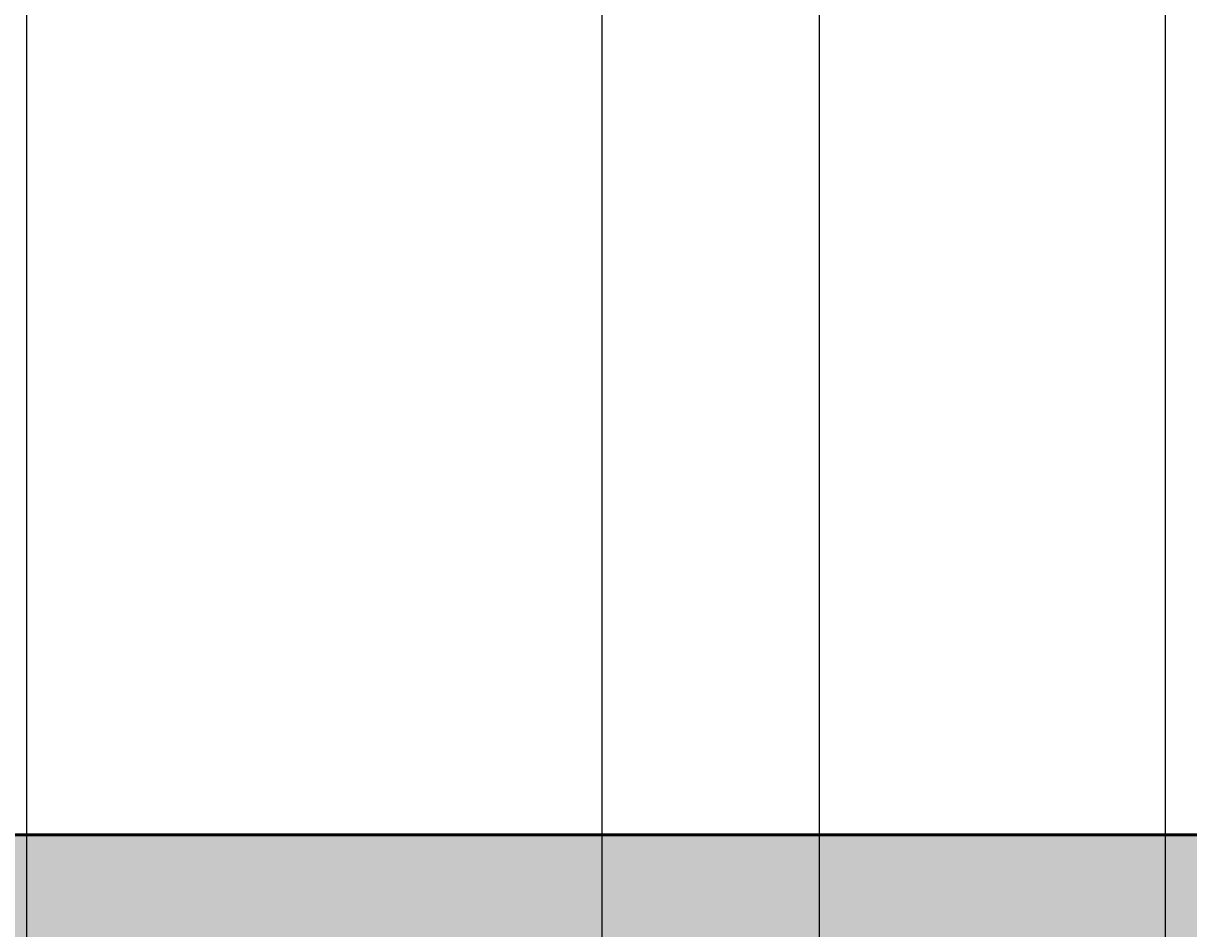
# Model space of a CAD drawing. Units: inches. Extents: x 2231 to 2461, y 2045 to 2455.
# Tile 81 of 95: x 2384 to 2409, y 2333 to 2352. Entities that reach past the tile are written whole.
import ezdxf

# ---------------------------------------------------------------- set-up
doc = ezdxf.new("R2010")
doc.units = ezdxf.units.IN
doc.layers.add('A-ANNO-DIMS', color=2, linetype='Continuous', lineweight=18)
doc.layers.add('A-WALL', color=7, linetype='Continuous', lineweight=50)
doc.layers.add('A-WALL-PATT', color=18, linetype='Continuous', lineweight=13, true_color=0x000000)
doc.styles.get("Standard").update_dxf_attribs({"font": 'arial.ttf'})
doc.dimstyles.get("Standard").update_dxf_attribs({"dimtxt": 0.18, "dimasz": 0.18, "dimexe": 0.18, "dimexo": 0.0625, "dimgap": 0.09, "dimtad": 0, "dimtih": 1, "dimtoh": 1, "dimdec": 4, "dimzin": 0, "dimdsep": 46, "dimtxsty": 'Standard', "dimcen": 0.09, "dimadec": 0, "dimazin": 0, "dimtfac": 1, "dimtdec": 4, "dimtofl": 0, "dimtmove": 0, "dimatfit": 3, "dimfxl": 1, "dimtolj": 1, "dimtzin": 0, "dimarcsym": 0})

# ---------------------------------------------------------------- blocks, each defined once
blk = doc.blocks.new('*D42')
at = {"layer": 'A-ANNO-DIMS', "color": 0, "lineweight": -2, "transparency": 16777216}
for p, q in [((2396.794, 2286.895), (2396.794, 2454.645)), ((2432.794, 2286.895), (2432.794, 2454.645)), ((2396.974, 2454.465), (2414.575, 2454.465)), ((2432.614, 2454.465), (2415.012, 2454.465))]:
    blk.add_line(p, q, dxfattribs=at)
at = {"layer": 'A-ANNO-DIMS', "color": 0, "transparency": 16777216}
for points in [[(2396.974, 2454.495), (2396.974, 2454.435), (2396.794, 2454.465)], [(2432.614, 2454.495), (2432.614, 2454.435), (2432.794, 2454.465)]]:
    blk.add_solid(points, dxfattribs=at)
at = {"layer": 'Defpoints', "color": 0, "transparency": 16777216}
for p in [(2432.794, 2454.465), (2396.794, 2286.833), (2432.794, 2286.833)]:
    blk.add_point(p, dxfattribs=at)
at = {"layer": 'A-ANNO-DIMS', "color": 0, "transparency": 16777216, "insert": (2414.794, 2454.465), "char_height": 0.18, "attachment_point": 5}
blk.add_mtext('\\A1;36', dxfattribs=at)
blk = doc.blocks.new('*D59')
at = {"layer": 'A-ANNO-DIMS', "color": 0, "lineweight": -2, "transparency": 16777216}
for p, q in [((2408.794, 2182.895), (2408.794, 2454.645)), ((2432.794, 2182.895), (2432.794, 2454.645)), ((2408.974, 2454.465), (2420.573, 2454.465)), ((2432.614, 2454.465), (2421.014, 2454.465))]:
    blk.add_line(p, q, dxfattribs=at)
at = {"layer": 'A-ANNO-DIMS', "color": 0, "transparency": 16777216}
for points in [[(2408.974, 2454.495), (2408.974, 2454.435), (2408.794, 2454.465)], [(2432.614, 2454.495), (2432.614, 2454.435), (2432.794, 2454.465)]]:
    blk.add_solid(points, dxfattribs=at)
at = {"layer": 'Defpoints', "color": 0, "transparency": 16777216}
for p in [(2432.794, 2454.465), (2408.794, 2182.833), (2432.794, 2182.833)]:
    blk.add_point(p, dxfattribs=at)
at = {"layer": 'A-ANNO-DIMS', "color": 0, "transparency": 16777216, "insert": (2420.794, 2454.465), "char_height": 0.18, "attachment_point": 5}
blk.add_mtext('\\A1;24', dxfattribs=at)
blk = doc.blocks.new('*D66')
at = {"layer": 'A-ANNO-DIMS', "color": 0, "lineweight": -2, "transparency": 16777216}
for p, q in [((2348.189, 2096.895), (2348.189, 2454.645)), ((2408.794, 2096.895), (2408.794, 2454.645)), ((2348.369, 2454.465), (2378.167, 2454.465)), ((2408.614, 2454.465), (2378.815, 2454.465))]:
    blk.add_line(p, q, dxfattribs=at)
at = {"layer": 'A-ANNO-DIMS', "color": 0, "transparency": 16777216}
for points in [[(2348.369, 2454.495), (2348.369, 2454.435), (2348.189, 2454.465)], [(2408.614, 2454.495), (2408.614, 2454.435), (2408.794, 2454.465)]]:
    blk.add_solid(points, dxfattribs=at)
at = {"layer": 'Defpoints', "color": 0, "transparency": 16777216}
for p in [(2408.794, 2454.465), (2348.189, 2096.833), (2408.794, 2096.833)]:
    blk.add_point(p, dxfattribs=at)
at = {"layer": 'A-ANNO-DIMS', "color": 0, "transparency": 16777216, "insert": (2378.491, 2454.465), "char_height": 0.18, "attachment_point": 5}
blk.add_mtext('\\A1;60.6', dxfattribs=at)
blk = doc.blocks.new('*D71')
at = {"layer": 'A-ANNO-DIMS', "color": 0, "lineweight": -2, "transparency": 16777216}
for p, q in [((2401.422, 2092.979), (2401.422, 2454.645)), ((2408.794, 2096.895), (2408.794, 2454.645)), ((2401.602, 2454.465), (2404.732, 2454.465)), ((2408.614, 2454.465), (2405.483, 2454.465))]:
    blk.add_line(p, q, dxfattribs=at)
at = {"layer": 'A-ANNO-DIMS', "color": 0, "transparency": 16777216}
for points in [[(2401.602, 2454.495), (2401.602, 2454.435), (2401.422, 2454.465)], [(2408.614, 2454.495), (2408.614, 2454.435), (2408.794, 2454.465)]]:
    blk.add_solid(points, dxfattribs=at)
at = {"layer": 'Defpoints', "color": 0, "transparency": 16777216}
for p in [(2408.794, 2454.465), (2408.794, 2096.833), (2401.422, 2092.917)]:
    blk.add_point(p, dxfattribs=at)
at = {"layer": 'A-ANNO-DIMS', "color": 0, "transparency": 16777216, "insert": (2405.108, 2454.465), "char_height": 0.18, "attachment_point": 5}
blk.add_mtext('\\A1;7.371', dxfattribs=at)
blk = doc.blocks.new('*D72')
at = {"layer": 'A-ANNO-DIMS', "color": 0, "lineweight": -2, "transparency": 16777216}
for p, q in [((2384.543, 2145.12), (2384.543, 2454.645)), ((2408.794, 2150.677), (2408.794, 2454.645)), ((2384.723, 2454.465), (2396.272, 2454.465)), ((2408.614, 2454.465), (2397.064, 2454.465))]:
    blk.add_line(p, q, dxfattribs=at)
at = {"layer": 'A-ANNO-DIMS', "color": 0, "transparency": 16777216}
for points in [[(2384.723, 2454.495), (2384.723, 2454.435), (2384.543, 2454.465)], [(2408.614, 2454.495), (2408.614, 2454.435), (2408.794, 2454.465)]]:
    blk.add_solid(points, dxfattribs=at)
at = {"layer": 'Defpoints', "color": 0, "transparency": 16777216}
for p in [(2408.794, 2454.465), (2408.794, 2150.615), (2384.543, 2145.058)]:
    blk.add_point(p, dxfattribs=at)
at = {"layer": 'A-ANNO-DIMS', "color": 0, "transparency": 16777216, "insert": (2396.668, 2454.465), "char_height": 0.18, "attachment_point": 5}
blk.add_mtext('\\A1;24.25', dxfattribs=at)

msp = doc.modelspace()

# ---------------------------------------------------------------- hatches: boundary and pattern name
at = {"layer": 'A-WALL-PATT'}
h = msp.add_hatch(color=256, dxfattribs=at)
h.dxf.hatch_style = 1
h.paths.add_polyline_path([(2441.7935, 2269.1535), (2432.7935, 2269.1535), (2432.7935, 2186.8328), (2396.7935, 2186.8328), (2396.7935, 2286.8328), (2394.7935, 2286.8328), (2394.7935, 2186.8328), (2334.7935, 2186.8328), (2334.7935, 2182.8328), (2432.7935, 2182.8328), (2432.7935, 2072.8328), (2416.6639, 2072.8328), (2416.6639, 2063.8328), (2441.7935, 2063.8328)])
h.paths.add_polyline_path([(2368.6639, 2072.8328), (2367.04, 2072.8328), (2330.7942, 2072.8328), (2330.7397, 2063.8328), (2368.6639, 2063.8328)])
h.paths.add_polyline_path([(2300.7392, 2068.3328), (2300.7392, 2072.8328), (2298.7935, 2072.8328), (2294.7935, 2072.8328), (2258.7935, 2072.8328), (2258.7935, 2120.8328), (2294.7935, 2120.8328), (2298.7935, 2120.8328), (2298.7935, 2128.8328), (2294.7935, 2128.8328), (2294.7935, 2124.8328), (2258.7935, 2124.8328), (2258.7935, 2182.8328), (2294.7935, 2182.8328), (2294.7935, 2174.8328), (2298.7935, 2174.8328), (2298.7935, 2182.8328), (2304.7935, 2182.8328), (2304.7935, 2186.8328), (2258.7935, 2186.8328), (2258.7935, 2221.999), (2249.7935, 2221.999), (2249.7935, 2063.8328), (2300.7392, 2063.8328)])
h.paths.add_polyline_path([(2391.9338, 2435.8328), (2333.82, 2435.8328), (2333.82, 2426.8328), (2368.7935, 2426.8328), (2368.7935, 2374.9508), (2368.7935, 2370.8328), (2372.3935, 2370.8328), (2372.7935, 2370.8328), (2372.7935, 2426.8328), (2391.9338, 2426.8328)])
h.paths.add_polyline_path([(2441.7935, 2435.8328), (2415.9338, 2435.8328), (2415.9338, 2426.8328), (2432.7935, 2426.8328), (2432.7935, 2334.8328), (2372.7935, 2334.8328), (2372.7935, 2346.8328), (2368.7935, 2346.8328), (2368.7935, 2306.8328), (2360.7935, 2306.8328), (2360.7935, 2302.8328), (2368.7935, 2302.8328), (2372.7935, 2302.8328), (2372.7935, 2330.8328), (2432.7935, 2330.8328), (2432.7935, 2317.1535), (2441.7935, 2317.1535)])
h.paths.add_polyline_path([(2285.82, 2435.8328), (2249.7935, 2435.8328), (2249.7935, 2269.999), (2258.7935, 2269.999), (2258.7935, 2302.8328), (2318.8168, 2302.8328), (2330.7935, 2302.8328), (2330.7935, 2306.8328), (2258.7935, 2306.8328), (2258.7935, 2426.8328), (2285.82, 2426.8328)])

# ---------------------------------------------------------------- linework, layer by layer
at = {"layer": 'A-WALL'}
msp.add_line((2372.7935, 2334.8328), (2432.7935, 2334.8328), dxfattribs=at)

# ---------------------------------------------------------------- dimensions: what is measured, and where the dimension line sits
at = {"layer": 'A-ANNO-DIMS'}
for base, p1, p2, override, picture, middle in [((2408.7935, 2454.4653), (2348.1888, 2096.8328), (2408.7935, 2096.8328), {"dimdec": 1, "dimlfac": 1, "dimrnd": 0, "dimzin": 0, "dimdsep": 46, "dimlunit": 2}, '*D66', (2378.4912, 2454.4653)), ((2408.7935, 2454.4653), (2384.5428, 2145.0576), (2408.7935, 2150.6145), {"dimdec": 2, "dimlfac": 1, "dimrnd": 0, "dimzin": 0, "dimdsep": 46, "dimlunit": 2}, '*D72', (2396.6682, 2454.4653)), ((2432.7935, 2454.4653), (2396.7935, 2286.8328), (2432.7935, 2286.8328), {"dimdec": 0, "dimlfac": 1, "dimrnd": 0, "dimzin": 0, "dimdsep": 46, "dimlunit": 2}, '*D42', (2414.7935, 2454.4653)), ((2408.7935, 2454.4653), (2401.4221, 2092.9167), (2408.7935, 2096.8328), {"dimdec": 3, "dimlfac": 1, "dimrnd": 0, "dimzin": 0, "dimdsep": 46, "dimlunit": 2}, '*D71', (2405.1078, 2454.4653)), ((2432.7935, 2454.4653), (2408.7935, 2182.8328), (2432.7935, 2182.8328), {"dimdec": 0, "dimlfac": 1, "dimrnd": 0, "dimzin": 0, "dimdsep": 46, "dimlunit": 2}, '*D59', (2420.7935, 2454.4653))]:
    dim = msp.add_linear_dim(base=base, p1=p1, p2=p2, dimstyle='Standard', override=override, dxfattribs=at)
    dim.commit()
    dim.dimension.update_dxf_attribs({"geometry": picture, "text_midpoint": middle})

doc.saveas('drawing.dxf')
